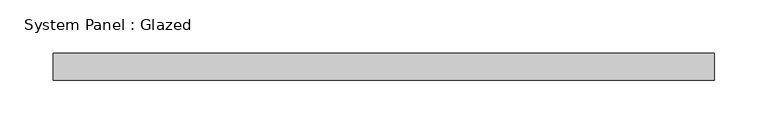
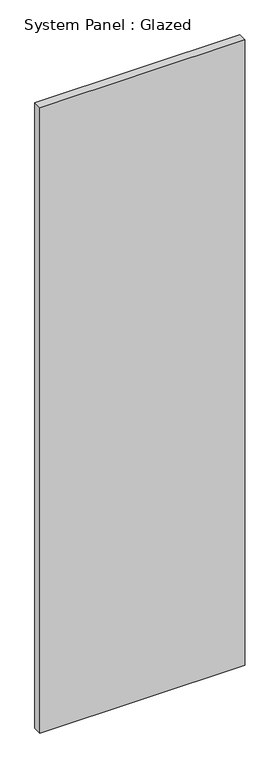
"""IFC4 building model written with IfcOpenShell, lengths in millimetres: plate geometry, System Panel : Glazed."""

from ifc_helpers import new_model, si_unit, origin, origin_with_axes, place, context, project, spatial, polyline, outline, extrude, source, transform, mapped, element, save


def system_panel_glazed_550f7026(model_context):
    return source(origin(), model_context, "Body", "SweptSolid", [
        extrude(outline(polyline([(311.15, 19.05), (-311.15, 19.05), (-311.15, 44.45), (311.15, 44.45), (311.15, 19.05)])), origin_with_axes(), (0.0, 0.0, 1.0), 2006.6),
    ])


if __name__ == "__main__":
    model = new_model("IFC4")
    model_context = context("Model", 3, world=origin())
    ifc_project = project(units=[si_unit("LENGTHUNIT", "METRE", prefix="MILLI")], contexts=[model_context])
    site = spatial("IfcSite", under=ifc_project)
    building = spatial("IfcBuilding", under=site)
    placement = place(None, origin())
    system_panel_glazed_shape = system_panel_glazed_550f7026(model_context)
    element("IfcPlate", 1, ObjectType="System Panel : Glazed", at=placement, inside=building, context=model_context, shape_type="MappedRepresentation", body=[
        mapped(system_panel_glazed_shape, transform((0.0, 0.0, 0.0), x_axis=(1.0, 0.0, 0.0), y_axis=(0.0, 1.0, 0.0), z_axis=(0.0, 0.0, 1.0))),
    ])
    save(model, "model.ifc")

# Revit data of these elements
# Type "System Panel : Glazed"
#   Construction Type Id = "GSP4R"
#   Analytic Construction = "1/8 in Pilkington single glazing"
#   Visual Light Transmittance = 0.9
#   Solar Heat Gain Coefficient = 0.86
#   Heat Transfer Coefficient (U) = 1.18115 BTU/(h·ft²·°F)
#   Define Thermal Properties by = 1
# Element 1 (IfcPlate, "System Panel : Glazed")
#   Materials on its faces: "Glass"
# Materials
#   "Glass": class "Glass", colour RGB 0 128 192, transparency 0.75, Description = "Soda Lime Glass", Cost = 0
